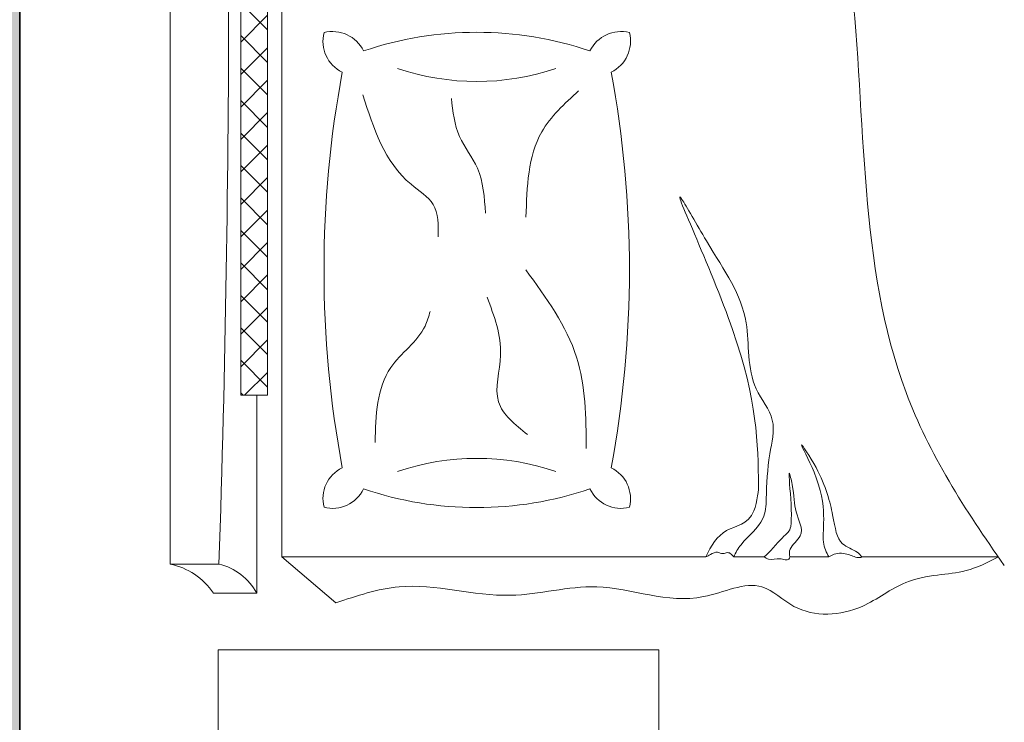
# Model space of a CAD drawing. Units: inches. Extents: x 2083 to 3317, y 1141 to 2115.
# Tile 95 of 256: x 2236 to 2290, y 1894 to 1932. Entities that reach past the tile are written whole.
import ezdxf

# ---------------------------------------------------------------- set-up
doc = ezdxf.new("R2010")
doc.units = ezdxf.units.IN
for name, color, linetype, lineweight in [('A-FURN', 8, 'Continuous', 18), ('A-WALL', 7, 'Continuous', 35), ('www.cadblocksfree.com', 7, 'Continuous', 9)]:
    doc.layers.add(name, color=color, linetype=linetype, lineweight=lineweight)
doc.layers.add('A-WALL-PATT', color=251, linetype='Continuous', lineweight=13, true_color=0x636466)

# ---------------------------------------------------------------- blocks, each defined once
blk = doc.blocks.new('bed')
at = {"layer": 'www.cadblocksfree.com', "ltscale": 0.2}
h = blk.add_hatch(dxfattribs=at)
h.set_pattern_fill('ANSI37,_O', color=256, scale=0.393701)
h.set_pattern_definition([(45, (2420.7222, -262.9689), (-0.8838835, 0.8838835), []), (135, (2420.7222, -262.9689), (-0.8838835, -0.8838835), [])])
h.paths.add_polyline_path([(3417.573, 1472.402), (3372.192, 1472.402), (3372.192, 1470.941), (3417.573, 1470.941)])
for p, q in [((3363.002, 1473.586), (3363.002, 1476.249)), ((3372.192, 1472.402), (3417.573, 1472.402)), ((3372.192, 1470.941), (3372.192, 1472.402)), ((3372.192, 1470.941), (3417.573, 1470.941)), ((3363.387, 1470.154), (3360.883, 1467.22))]:
    blk.add_line(p, q, dxfattribs=at)
for points in [[(3426.763, 1476.249), (3363.002, 1476.249)], [(3361.418, 1473.886), (3361.418, 1471.524), (3372.192, 1471.524)], [(3426.379, 1449.413), (3426.379, 1470.154), (3363.387, 1470.154), (3363.387, 1447.076)], [(3363.387, 1445.539), (3363.387, 1443.892)], [(3363.387, 1442.495), (3363.387, 1440.369)], [(3363.387, 1438.564), (3363.387, 1431.137)]]:
    blk.add_lwpolyline(points, dxfattribs=at)
for centre, radius, start, end in [((3359.334, 1476.997), 3.744, 303.8271, 348.4775), ((3359.844, 1474.373), 3.255, 298.9176, 345.9939), ((3394.883, 2431.358), 958.303, 268.093559, 271.906441), ((3367.903, 1467.396), 1.87, 165.5166, 244.2099), ((3366.56, 1466.054), 1.87, 25.7901, 104.4834), ((3379.014, 1409.187), 58.677, 79.42346, 100.57654), ((3391.467, 1466.054), 1.87, 75.5166, 154.2099), ((3390.125, 1467.396), 1.87, 295.7901, 14.4834), ((3385.289, 1459.547), 19.215, 161.2852, 198.7148), ((3372.739, 1459.547), 19.215, 341.2852, 18.7148), ((3355.416, 1459.547), 13.338, 341.1598, 18.8402), ((3402.612, 1459.547), 13.338, 161.1598, 198.8402), ((3367.903, 1451.698), 1.87, 115.7901, 194.4834), ((3390.125, 1451.698), 1.87, 345.5166, 64.2099), ((3366.56, 1453.041), 1.87, 255.5166, 334.2099), ((3379.014, 1509.907), 58.677, 259.42346, 280.57654), ((3391.467, 1453.041), 1.87, 205.7901, 284.4834)]:
    blk.add_arc(centre, radius, start, end, dxfattribs=at)
for points, knots in [([(3360.883, 1467.22), (3361.272, 1466.08), (3362.328, 1462.983), (3360.73, 1458.154), (3362.389, 1452.621), (3360.35, 1448.139), (3362.429, 1444.241), (3360.039, 1441.931), (3360.256, 1438.678), (3362.05, 1436.545), (3362.42, 1434.517), (3362.566, 1432.758), (3363.096, 1431.712), (3363.387, 1431.137)], [0, 0, 0, 0, 3.550403, 9.643115, 14.356056, 20.206026, 23.427697, 25.46537, 29.172767, 31.884544, 33.668442, 35.237641, 37.145618, 37.145618, 37.145618, 37.145618]), ([(3388.545, 1465.744), (3386.719, 1465.161), (3384.357, 1464.407), (3382.678, 1461.635), (3381.454, 1461.638), (3380.813, 1461.64)], [0, 0, 0, 0, 5.530688, 7.154877, 8.940839, 8.940839, 8.940839, 8.940839]), ([(3369.625, 1465.083), (3371.104, 1465.041), (3373.625, 1464.969), (3375.264, 1462.52), (3376.483, 1462.165), (3376.755, 1462.086)], [0, 0, 0, 0, 4.163459, 7.093919, 7.934624, 7.934624, 7.934624, 7.934624]), ([(3388.358, 1460.927), (3387.639, 1460.846), (3386.254, 1460.689), (3384.483, 1459.224), (3382.96, 1459.127), (3382.112, 1459.073)], [0, 0, 0, 0, 2.127543, 4.10272, 6.58647, 6.58647, 6.58647, 6.58647]), ([(3370.049, 1456.774), (3370.592, 1457.459), (3371.713, 1458.876), (3374.682, 1457.893), (3376.505, 1458.594), (3377.525, 1458.985)], [0, 0, 0, 0, 2.388143, 4.935423, 8.166198, 8.166198, 8.166198, 8.166198]), ([(3369.287, 1453.579), (3370.996, 1453.599), (3374.587, 1453.639), (3377.497, 1455.762), (3379.021, 1456.874)], [0, 0, 0, 0, 5.002087, 10.507046, 10.507046, 10.507046, 10.507046]), ([(3388.77, 1453.995), (3388.068, 1454.761), (3386.268, 1456.726), (3383.544, 1456.811), (3381.881, 1456.863)], [0, 0, 0, 0, 3.013696, 7.735839, 7.735839, 7.735839, 7.735839]), ([(3367.269, 1444.201), (3369.575, 1444.23), (3373.917, 1444.284), (3385.471, 1449.8), (3379.558, 1446.493), (3376.808, 1444.477), (3372.948, 1444.924), (3370.926, 1443.14), (3368.771, 1443.702), (3367.359, 1443.752), (3366.554, 1443.781)], [0, 0, 0, 0, 8.61026, 16.221274, 18.843057, 23.804898, 27.440828, 29.356102, 31.203478, 33.650687, 33.650687, 33.650687, 33.650687]), ([(3363.387, 1447.076), (3363.429, 1446.99), (3363.529, 1446.784), (3363.731, 1446.461), (3363.506, 1446.154), (3363.665, 1445.905), (3363.559, 1445.673), (3363.444, 1445.584), (3363.387, 1445.539)], [0, 0, 0, 0, 0.293454, 0.701471, 1.003873, 1.254893, 1.47342, 1.69185, 1.69185, 1.69185, 1.69185]), ([(3363.387, 1447.076), (3363.991, 1446.782), (3365.084, 1446.124), (3365.119, 1444.371), (3367.129, 1444.191), (3367.269, 1444.201)], [0.0122268, 0.0122268, 0.0122268, 0.0122268, 0.0594721, 0.1062177, 0.134458, 0.134458, 0.134458, 0.134458]), ([(3366.554, 1443.781), (3366.17, 1443.775), (3365.174, 1443.901), (3364.4, 1444.957), (3363.626, 1445.461), (3363.387, 1445.539)], [0.15648839, 0.15648839, 0.15648839, 0.15648839, 0.18439755, 0.23137648, 0.25059846, 0.25059846, 0.25059846, 0.25059846]), ([(3363.387, 1443.892), (3363.335, 1443.815), (3363.165, 1443.56), (3363.346, 1443.124), (3363.233, 1442.791), (3363.225, 1442.533), (3363.341, 1442.506), (3363.387, 1442.495)], [0, 0, 0, 0, 0.27176, 0.887321, 1.189132, 1.388142, 1.515331, 1.515331, 1.515331, 1.515331]), ([(3363.387, 1443.892), (3363.631, 1443.61), (3364.671, 1442.733), (3364.886, 1442.149), (3369.073, 1442.744), (3366.773, 1442.243), (3365.832, 1442.298), (3364.615, 1441.552), (3363.961, 1442.542), (3363.537, 1442.524), (3363.387, 1442.495)], [0.0595743, 0.0595743, 0.0595743, 0.0595743, 0.0807529, 0.1037415, 0.1697201, 0.1760361, 0.2071372, 0.2404744, 0.2623409, 0.2736605, 0.2736605, 0.2736605, 0.2736605]), ([(3362.928, 1430.813), (3365.944, 1432.958), (3375.455, 1438.993), (3392.12, 1438.03), (3404.249, 1440.73), (3408.408, 1442.961)], [0.102872, 0.102872, 0.102872, 0.102872, 0.37972, 0.957702, 1.313793, 1.313793, 1.313793, 1.313793]), ([(3363.387, 1440.369), (3363.634, 1440.51), (3364.527, 1440.899), (3366.485, 1440.246), (3370.203, 1442.295), (3367.731, 1440.636), (3365.42, 1440.07), (3364.035, 1439.913), (3363.795, 1438.935), (3363.482, 1438.64), (3363.387, 1438.564)], [0.013856, 0.013856, 0.013856, 0.013856, 0.0348738, 0.0888667, 0.1078792, 0.1267378, 0.158714, 0.1937575, 0.2174868, 0.2267221, 0.2267221, 0.2267221, 0.2267221]), ([(3363.387, 1440.369), (3363.445, 1440.274), (3363.571, 1440.065), (3363.607, 1439.678), (3363.531, 1439.31), (3363.405, 1439.003), (3363.329, 1438.751), (3363.372, 1438.611), (3363.387, 1438.564)], [0, 0, 0, 0, 0.329977, 0.725302, 1.129072, 1.442831, 1.734218, 1.878348, 1.878348, 1.878348, 1.878348])]:
    blk.add_open_spline(points, degree=3, knots=knots, dxfattribs=at)

msp = doc.modelspace()

# ---------------------------------------------------------------- hatches: boundary and pattern name
at = {"layer": 'A-WALL-PATT'}
h = msp.add_hatch(color=256, dxfattribs=at)
h.dxf.hatch_style = 1
h.paths.add_polyline_path([(3126.96, 2020.761), (2748.96, 2020.761), (2604.96, 2020.761), (2226.96, 2020.761), (2226.96, 1702.761), (2466.96, 1702.761), (2466.96, 1582.761), (2418.96, 1582.761), (2418.96, 1477.761), (2226.96, 1477.761), (2226.96, 1263.261), (2544.96, 1263.261), (2544.96, 1411.761), (2604.96, 1411.761), (2685.96, 1411.761), (2685.96, 1420.761), (2604.96, 1420.761), (2604.96, 1573.761), (2604.96, 1702.761), (2604.96, 2011.761), (2748.96, 2011.761), (2748.96, 1702.761), (2862.96, 1702.761), (2862.96, 1621.761), (2871.96, 1621.761), (2871.96, 1702.761), (2883.96, 1702.761), (2883.96, 1706.939, -0.026459), (2883.96, 1711.761), (2757.96, 1711.761), (2757.96, 1807.761), (2787.96, 1807.761), (2787.96, 1812.261), (2757.96, 1812.261), (2757.96, 2011.761), (2877.96, 2011.761), (2877.96, 1812.261), (2847.96, 1812.261), (2847.96, 1807.761), (2889.836, 1807.761), (2889.836, 1812.261), (2882.46, 1812.261), (2882.46, 2011.761), (3117.96, 2011.761), (3117.96, 1812.261), (2937.836, 1812.261), (2937.836, 1807.761), (2995.71, 1807.761), (2995.71, 1796.118), (3000.21, 1796.118), (3000.21, 1807.761), (3117.96, 1807.761), (3117.96, 1711.761), (3000.21, 1711.761), (3000.21, 1760.118), (2998.573, 1760.118, -0.020711), (2995.71, 1760.118), (2995.71, 1711.761), (2931.96, 1711.761), (2931.96, 1702.761), (3126.96, 1702.761)])
h.paths.add_polyline_path([(2471.46, 2011.761), (2471.46, 1810.011), (2462.717, 1810.011), (2462.717, 1805.511), (2505.96, 1805.511), (2505.96, 1810.011), (2475.96, 1810.011), (2475.96, 2011.761), (2595.96, 2011.761), (2595.96, 1810.011), (2565.96, 1810.011), (2565.96, 1805.511), (2595.96, 1805.511), (2595.96, 1711.761), (2235.96, 1711.761), (2235.96, 1805.511), (2353.71, 1805.511), (2353.71, 1796.054), (2358.21, 1796.054), (2358.21, 1805.511), (2414.717, 1805.511), (2414.717, 1810.011), (2235.96, 1810.011), (2235.96, 2011.761)], flags=16)
h.paths.add_polyline_path([(2270.205, 1994.61), (2270.205, 1970.61), (2246.205, 1970.61), (2246.205, 1994.61)], flags=0)
edge = h.paths.add_edge_path(flags=0)
edge.add_ellipse((2332.027, 1899.798), major_axis=(-3.043, 3.043), ratio=0.168252, start_angle=-161.3322, end_angle=-156.3071, ccw=False)
edge.add_ellipse((2333.082, 1898.744), major_axis=(-1.055, 1.055), ratio=0.453532, start_angle=-123.371, end_angle=-94.1591)
edge = h.paths.add_edge_path(flags=0)
edge.add_ellipse((2332.027, 1968.876), major_axis=(3.043, 3.043), ratio=0.168252, start_angle=18.6678, end_angle=23.6929)
edge.add_spline(control_points=[(2332.926, 1970.691), (2332.227, 1970.336), (2330.894, 1969.659), (2328.413, 1970.932), (2327.204, 1967.749), (2324.71, 1969.956), (2322.533, 1967.012), (2320.013, 1971.296), (2317.68, 1968.158), (2316.041, 1967.102), (2315.427, 1966.81)], knot_values=[0, 0, 0, 0, 2.267059, 4.324559, 6.685584, 8.878641, 11.121502, 14.300359, 17.755284, 19.732645, 19.732645, 19.732645, 19.732645], degree=3, periodic=0)
edge.add_ellipse((2332.027, 1968.876), major_axis=(3.043, 3.043), ratio=0.168252, start_angle=18.6678, end_angle=23.6929, ccw=False)
edge.add_ellipse((2333.082, 1969.931), major_axis=(1.055, 1.055), ratio=0.453532, start_angle=56.629, end_angle=85.8409, ccw=False)
edge = h.paths.add_edge_path(flags=0)
edge.add_spline(control_points=[(2296.428, 1967.988), (2293.628, 1965.336), (2287.704, 1959.727), (2299.744, 1949.996), (2294.533, 1935.669), (2290.573, 1920.604), (2293.394, 1909.974), (2296.185, 1904.967)], knot_values=[0.099185, 0.099185, 0.099185, 0.099185, 0.345301, 0.619822, 0.982653, 1.386093, 1.810555, 1.810555, 1.810555, 1.810555], degree=3, periodic=0)
edge.add_spline(control_points=[(2296.185, 1904.967), (2297.384, 1902.619), (2298.001, 1901.949), (2298.553, 1901.468)], knot_values=[0.006246, 0.006246, 0.006246, 0.006246, 0.055476, 0.055476, 0.055476, 0.055476], degree=3, periodic=0)
edge.add_spline(control_points=[(2298.553, 1901.468), (2297.259, 1900.923), (2295.225, 1900.232), (2293.06, 1900.614), (2292.101, 1900.788), (2292.09, 1900.791)], knot_values=[0.312835, 0.312835, 0.312835, 0.312835, 0.40178, 0.474987, 0.475903, 0.475903, 0.475903, 0.475903], degree=3, periodic=0)
edge.add_arc((2292.794, 1904.664), 3.937, 215.4209, 259.6982, ccw=False)
edge.add_spline(control_points=[(2289.585, 1902.382), (2289.477, 1902.535), (2289.368, 1902.688), (2289.261, 1902.841)], knot_values=[0.102872, 0.102872, 0.102872, 0.102872, 0.116896, 0.116896, 0.116896, 0.116896], degree=3, periodic=0)
edge.add_spline(control_points=[(2289.261, 1902.841), (2288.687, 1902.55), (2287.64, 1902.02), (2285.881, 1901.874), (2283.853, 1901.504), (2281.72, 1899.711), (2278.467, 1899.493), (2276.157, 1901.883), (2272.259, 1899.804), (2267.778, 1901.843), (2262.244, 1900.184), (2257.415, 1901.782), (2254.318, 1900.726), (2253.178, 1900.337)], knot_values=[0, 0, 0, 0, 1.907977, 3.477176, 5.261074, 7.972851, 11.680248, 13.717921, 16.939592, 22.789562, 27.502503, 33.595215, 37.145618, 37.145618, 37.145618, 37.145618], degree=3, periodic=0)
edge.add_line((2253.178, 1900.337), (2250.244, 1902.841))
edge.add_line((2250.244, 1902.841), (2250.244, 1965.833))
edge.add_line((2250.244, 1965.833), (2253.178, 1968.337))
edge.add_spline(control_points=[(2253.178, 1968.337), (2254.318, 1967.948), (2257.415, 1966.892), (2262.244, 1968.49), (2267.778, 1966.831), (2271.527, 1968.537), (2273.876, 1967.828), (2274.207, 1967.728)], knot_values=[0, 0, 0, 0, 0.09018, 0.244935, 0.364644, 0.513233, 0.537855, 0.537855, 0.537855, 0.537855], degree=3, periodic=0)
edge.add_arc((2274.353, 1963.793), 3.937, 72.0511, 92.1279, ccw=False)
edge.add_arc((2281.297, 1985.23), 18.596, 252.0511, 288.5657)
edge.add_arc((2292.317, 1956.029), 12.646, 71.0268, 113.7782, ccw=False)
edge = h.paths.add_edge_path(flags=0)
edge.add_spline(control_points=[(2274.899, 1951.856), (2275.066, 1951.617), (2275.233, 1951.377), (2275.398, 1951.136)], knot_values=[1.409916, 1.409916, 1.409916, 1.409916, 1.43159, 1.43159, 1.43159, 1.43159], degree=3, periodic=0)
edge.add_spline(control_points=[(2275.398, 1951.136), (2275.792, 1950.562), (2276.179, 1949.984), (2276.546, 1949.397)], knot_values=[1.358238, 1.358238, 1.358238, 1.358238, 1.409916, 1.409916, 1.409916, 1.409916], degree=3, periodic=0)
edge.add_line((2276.546, 1949.397), (2277.437, 1947.862))
edge.add_spline(control_points=[(2277.437, 1947.862), (2276.304, 1945.673), (2274.64, 1942.427), (2274.632, 1938.094), (2272.799, 1930.852), (2274.356, 1943.897), (2275.948, 1947.923), (2276.546, 1949.397)], knot_values=[0.005632, 0.005632, 0.005632, 0.005632, 0.186014, 0.266002, 0.357087, 0.59639, 0.739732, 0.739732, 0.739732, 0.739732], degree=3, periodic=0)
edge.add_spline(control_points=[(2276.546, 1949.397), (2276.179, 1949.984), (2275.792, 1950.562), (2275.398, 1951.136)], knot_values=[1.358238, 1.358238, 1.358238, 1.358238, 1.409916, 1.409916, 1.409916, 1.409916], degree=3, periodic=0)
edge.add_spline(control_points=[(2275.398, 1951.136), (2274.943, 1950.08), (2274.208, 1948.025), (2273.935, 1944.851), (2272.469, 1937.627), (2273.466, 1945.696), (2274.701, 1951.059), (2274.899, 1951.856)], knot_values=[0.104364, 0.104364, 0.104364, 0.104364, 0.189636, 0.269624, 0.36071, 0.600013, 0.644622, 0.644622, 0.644622, 0.644622], degree=3, periodic=0)
h.paths.add_polyline_path([(2269.168, 1963.128, -0.357527), (2268.171, 1960.976, -0.092561), (2268.171, 1939.436, -0.357527), (2269.168, 1937.285, -0.357527), (2267.016, 1938.282, -0.164785), (2254.686, 1938.282, -0.357527), (2252.534, 1937.285, -0.357527), (2253.531, 1939.436, -0.092561), (2253.531, 1960.976, -0.357527), (2252.534, 1963.128, -0.357527), (2254.686, 1962.131, -0.164785), (2267.016, 1962.131, -0.357527)], flags=0)
h.paths.add_polyline_path([(2248.874, 1967.802), (2248.874, 1957.028), (2249.458, 1957.028), (2249.458, 1911.647), (2248.874, 1911.647), (2248.874, 1900.873), (2246.512, 1900.873, 0.197327), (2244.15, 1902.457), (2244.15, 1966.218, 0.197327), (2246.512, 1967.802)], flags=0)
h.paths.add_polyline_path([(2269.168, 1931.389, -0.357527), (2268.171, 1929.238, -0.092561), (2268.171, 1907.698, -0.357527), (2269.168, 1905.547, -0.357527), (2267.016, 1906.544, -0.164785), (2254.686, 1906.544, -0.357527), (2252.534, 1905.547, -0.357527), (2253.531, 1907.698, -0.092561), (2253.531, 1929.238, -0.357527), (2252.534, 1931.389, -0.357527), (2254.686, 1930.392, -0.164785), (2267.016, 1930.392, -0.357527)], flags=0)
edge = h.paths.add_edge_path(flags=0)
edge.add_spline(control_points=[(2276.197, 1906.724), (2276.168, 1909.029), (2276.114, 1913.372), (2270.598, 1924.925), (2273.905, 1919.013), (2275.922, 1916.262), (2275.475, 1912.402), (2277.258, 1910.381), (2276.696, 1908.225), (2276.646, 1906.813), (2276.618, 1906.008)], knot_values=[0, 0, 0, 0, 8.61026, 16.221274, 18.843057, 23.804898, 27.440828, 29.356102, 31.203478, 33.650687, 33.650687, 33.650687, 33.650687], degree=3, periodic=0)
edge.add_spline(control_points=[(2276.618, 1906.008), (2276.623, 1905.624), (2276.498, 1904.629), (2275.442, 1903.855), (2274.937, 1903.08), (2274.859, 1902.841)], knot_values=[0.156488, 0.156488, 0.156488, 0.156488, 0.184398, 0.231376, 0.250598, 0.250598, 0.250598, 0.250598], degree=3, periodic=0)
edge.add_line((2274.859, 1902.841), (2276.506, 1902.841))
edge.add_spline(control_points=[(2276.506, 1902.841), (2276.788, 1903.085), (2277.665, 1904.125), (2278.25, 1904.341), (2277.654, 1908.527), (2278.156, 1906.228), (2278.1, 1905.286), (2278.847, 1904.069), (2277.857, 1903.415), (2277.874, 1902.991), (2277.904, 1902.841)], knot_values=[0.059574, 0.059574, 0.059574, 0.059574, 0.080753, 0.103741, 0.16972, 0.176036, 0.207137, 0.240474, 0.262341, 0.27366, 0.27366, 0.27366, 0.27366], degree=3, periodic=0)
edge.add_line((2277.904, 1902.841), (2280.03, 1902.841))
edge.add_spline(control_points=[(2280.03, 1902.841), (2279.888, 1903.088), (2279.499, 1903.982), (2280.152, 1905.939), (2278.104, 1909.658), (2279.762, 1907.185), (2280.328, 1904.875), (2280.485, 1903.49), (2281.463, 1903.249), (2281.758, 1902.936), (2281.834, 1902.841)], knot_values=[0.013856, 0.013856, 0.013856, 0.013856, 0.034874, 0.088867, 0.107879, 0.126738, 0.158714, 0.193757, 0.217487, 0.226722, 0.226722, 0.226722, 0.226722], degree=3, periodic=0)
edge.add_spline(control_points=[(2281.834, 1902.841), (2281.788, 1902.827), (2281.647, 1902.783), (2281.396, 1902.859), (2281.088, 1902.985), (2280.721, 1903.061), (2280.333, 1903.026), (2280.125, 1902.899), (2280.03, 1902.841)], knot_values=[0, 0, 0, 0, 0.14413, 0.435517, 0.749276, 1.153046, 1.548371, 1.878348, 1.878348, 1.878348, 1.878348], degree=3, periodic=0)
edge.add_line((2280.03, 1902.841), (2277.904, 1902.841))
edge.add_spline(control_points=[(2277.904, 1902.841), (2277.893, 1902.796), (2277.865, 1902.68), (2277.607, 1902.687), (2277.274, 1902.801), (2276.838, 1902.62), (2276.584, 1902.789), (2276.506, 1902.841)], knot_values=[0, 0, 0, 0, 0.127189, 0.326199, 0.628009, 1.24357, 1.515331, 1.515331, 1.515331, 1.515331], degree=3, periodic=0)
edge.add_line((2276.506, 1902.841), (2274.859, 1902.841))
edge.add_spline(control_points=[(2274.859, 1902.841), (2274.814, 1902.899), (2274.725, 1903.013), (2274.493, 1903.119), (2274.244, 1902.961), (2273.937, 1903.185), (2273.614, 1902.983), (2273.408, 1902.883), (2273.322, 1902.841)], knot_values=[0, 0, 0, 0, 0.21843, 0.436957, 0.687977, 0.990379, 1.398396, 1.69185, 1.69185, 1.69185, 1.69185], degree=3, periodic=0)
edge.add_spline(control_points=[(2273.322, 1902.841), (2273.617, 1903.446), (2274.274, 1904.538), (2276.027, 1904.574), (2276.207, 1906.584), (2276.197, 1906.724)], knot_values=[0.012227, 0.012227, 0.012227, 0.012227, 0.059472, 0.106218, 0.134458, 0.134458, 0.134458, 0.134458], degree=3, periodic=0)
h.paths.add_polyline_path([(2270.776, 1897.79), (2270.776, 1873.79), (2246.776, 1873.79), (2246.776, 1897.79)], flags=0)
h.paths.add_polyline_path([(2353.71, 1760.005), (2353.71, 1760.054), (2358.21, 1760.054, -0.033729)], flags=0)
h.paths.add_polyline_path([(2321.819, 1737.529), (2341.995, 1737.529, -0.414214), (2343.203, 1736.321), (2343.203, 1721.021, -0.414214), (2341.995, 1719.813), (2321.819, 1719.813, -0.414214), (2320.611, 1721.021), (2320.611, 1736.321, -0.414214)], flags=0)
h.paths.add_polyline_path([(2324.235, 1736.321), (2339.579, 1736.321, -0.414214), (2341.995, 1733.905), (2341.995, 1725.45, -0.414214), (2339.579, 1723.034), (2333.681, 1723.034), (2333.845, 1722.045, -0.870646), (2335.425, 1721.826, -0.767327), (2333.923, 1721.423), (2331.291, 1721.423, -0.767327), (2329.788, 1721.826, -0.870646), (2331.368, 1722.045), (2331.533, 1723.034), (2324.235, 1723.034, -0.414214), (2321.819, 1725.45), (2321.819, 1733.905, -0.414214)], flags=0)
h.paths.add_polyline_path([(2570.484, 1928.615), (2589.684, 1928.615), (2590.169, 1928.615), (2590.169, 1904.993), (2570.484, 1904.993)], flags=0)
h.paths.add_polyline_path([(2574.447, 1927.264, -1), (2572.829, 1927.264, -1)], flags=0)
h.paths.add_polyline_path([(2573.09, 1926.941), (2573.925, 1927.776), (2574.148, 1927.553), (2573.313, 1926.718)], flags=0)
h.paths.add_polyline_path([(2578.779, 1919.73, -1), (2571.592, 1919.73, -1)], flags=0)
h.paths.add_polyline_path([(2578.385, 1919.73, -1), (2571.985, 1919.73, -1)], flags=0)
h.paths.add_polyline_path([(2331.596, 1729.476, -1), (2333.618, 1729.476, -1)], flags=0)
h.paths.add_polyline_path([(2578.034, 1927.264, -1), (2576.416, 1927.264, -1)], flags=0)
h.paths.add_polyline_path([(2576.689, 1927.531), (2576.912, 1927.754), (2577.747, 1926.919), (2577.524, 1926.696)], flags=0)
h.paths.add_polyline_path([(2578.139, 1909.86, -1), (2572.232, 1909.86, -1)], flags=0)
h.paths.add_polyline_path([(2577.745, 1909.86, -1), (2572.625, 1909.86, -1)], flags=0)
h.paths.add_polyline_path([(2583.798, 1927.264, -1), (2582.179, 1927.264, -1)], flags=0)
h.paths.add_polyline_path([(2582.719, 1927.754), (2583.554, 1926.919), (2583.331, 1926.696), (2582.496, 1927.531)], flags=0)
h.paths.add_polyline_path([(2582.496, 1927.531), (2582.719, 1927.754), (2583.554, 1926.919), (2583.331, 1926.696)], flags=0)
h.paths.add_polyline_path([(2587.739, 1920.53, -1), (2581.832, 1920.53, -1)], flags=0)
h.paths.add_polyline_path([(2587.345, 1920.53, -1), (2582.225, 1920.53, -1)], flags=0)
h.paths.add_polyline_path([(2587.385, 1927.264, -1), (2585.766, 1927.264, -1)], flags=0)
h.paths.add_polyline_path([(2586.082, 1926.98), (2586.917, 1927.815), (2587.14, 1927.593), (2586.305, 1926.758)], flags=0)
h.paths.add_polyline_path([(2588.379, 1910.66, -1), (2581.192, 1910.66, -1)], flags=0)
h.paths.add_polyline_path([(2587.985, 1910.66, -1), (2581.585, 1910.66, -1)], flags=0)
h.paths.add_polyline_path([(2417.168, 1729.478), (2437.344, 1729.478, -0.414214), (2438.552, 1728.27), (2438.552, 1712.969, -0.414214), (2437.344, 1711.761), (2417.168, 1711.761, -0.414214), (2415.96, 1712.969), (2415.96, 1728.27, -0.414214)], flags=0)
h.paths.add_polyline_path([(2419.584, 1728.27), (2434.928, 1728.27, -0.414214), (2437.344, 1725.854), (2437.344, 1717.398, -0.414214), (2434.928, 1714.983), (2429.029, 1714.983), (2429.194, 1713.994, -0.870646), (2430.774, 1713.775, -0.767327), (2429.271, 1713.372), (2426.64, 1713.372, -0.767327), (2425.137, 1713.775, -0.870646), (2426.717, 1713.994), (2426.882, 1714.983), (2419.584, 1714.983, -0.414214), (2417.168, 1717.398), (2417.168, 1725.854, -0.414214)], flags=0)
h.paths.add_polyline_path([(2419.584, 1728.27), (2434.928, 1728.27, -0.414214), (2437.344, 1725.854), (2437.344, 1717.398, -0.414214), (2434.928, 1714.983), (2429.029, 1714.983), (2428.358, 1719.009), (2427.553, 1719.009), (2426.882, 1714.983), (2419.584, 1714.983, -0.414214), (2417.168, 1717.398), (2417.168, 1725.854, -0.414214)], flags=0)
h.paths.add_polyline_path([(2426.944, 1721.425, -1), (2428.967, 1721.425, -1)], flags=0)
h.paths.add_polyline_path([(2475.96, 1702.761), (2595.96, 1702.761), (2595.96, 1582.761), (2475.96, 1582.761)], flags=16)
h.paths.add_polyline_path([(2427.96, 1573.761), (2595.96, 1573.761), (2595.96, 1468.761), (2595.96, 1420.761), (2384.46, 1420.761), (2384.46, 1468.761), (2427.96, 1468.761)], flags=16)
h.paths.add_polyline_path([(2379.96, 1468.761), (2379.96, 1420.761), (2235.96, 1420.761), (2235.96, 1468.761)], flags=16)
h.paths.add_polyline_path([(2317.816, 1466.696), (2337.992, 1466.696, -0.414214), (2339.2, 1465.488), (2339.2, 1450.187, -0.414214), (2337.992, 1448.979), (2317.816, 1448.979, -0.414214), (2316.608, 1450.187), (2316.608, 1465.488, -0.414214)], flags=0)
h.paths.add_polyline_path([(2320.232, 1465.488), (2335.576, 1465.488, -0.414214), (2337.992, 1463.072), (2337.992, 1454.616, -0.414214), (2335.576, 1452.2), (2329.677, 1452.2), (2329.842, 1451.212, -0.870646), (2331.422, 1450.992, -0.767327), (2329.92, 1450.59), (2327.288, 1450.59, -0.767327), (2325.785, 1450.992, -0.870646), (2327.365, 1451.212), (2327.53, 1452.2), (2320.232, 1452.2, -0.414214), (2317.816, 1454.616), (2317.816, 1463.072, -0.414214)], flags=0)
h.paths.add_polyline_path([(2320.232, 1465.488), (2335.576, 1465.488, -0.414214), (2337.992, 1463.072), (2337.992, 1454.616, -0.414214), (2335.576, 1452.2), (2329.677, 1452.2), (2329.006, 1456.227), (2328.201, 1456.227), (2327.53, 1452.2), (2320.232, 1452.2, -0.414214), (2317.816, 1454.616), (2317.816, 1463.072, -0.414214)], flags=0)
h.paths.add_polyline_path([(2327.593, 1458.643, -1), (2329.615, 1458.643, -1)], flags=0)
h.paths.add_polyline_path([(2244.412, 1433.34), (2241.921, 1433.34, -0.414214), (2240.018, 1435.244), (2240.018, 1440.953, -0.414211), (2241.921, 1442.856), (2244.412, 1442.856, -1.976472)], flags=0)
h.paths.add_polyline_path([(2245.357, 1434.398, -0.414214), (2245.357, 1441.799, -2.144098)], flags=0)
h.paths.add_polyline_path([(2535.96, 1416.261), (2535.96, 1272.261), (2235.96, 1272.261), (2235.96, 1416.261)], flags=16)
h.paths.add_polyline_path([(2260.12, 1384.293), (2260.12, 1362.039), (2237.865, 1362.039), (2237.865, 1384.293)], flags=0)
edge = h.paths.add_edge_path(flags=0)
edge.add_line((2318.252, 1362.093), (2318.146, 1362.001))
edge.add_ellipse((2317.445, 1360.431), major_axis=(2.822, 2.822), ratio=0.168252, start_angle=18.6678, end_angle=20.9481, ccw=False)
edge.add_ellipse((2318.423, 1361.409), major_axis=(0.978, 0.978), ratio=0.453532, start_angle=56.629, end_angle=70.2262, ccw=False)
edge = h.paths.add_edge_path(flags=0)
edge.add_line((2319.107, 1295.571), (2319.015, 1295.677))
edge.add_ellipse((2317.445, 1296.378), major_axis=(-2.822, 2.822), ratio=0.168252, start_angle=-161.3322, end_angle=-159.0519, ccw=False)
edge.add_ellipse((2318.423, 1295.4), major_axis=(-0.978, 0.978), ratio=0.453532, start_angle=-123.371, end_angle=-109.7738)
edge = h.paths.add_edge_path(flags=0)
edge.add_spline(control_points=[(2284.21, 1301.17), (2284.581, 1300.445), (2284.891, 1299.892), (2285.16, 1299.461)], knot_values=[0.039066, 0.039066, 0.039066, 0.039066, 0.055476, 0.055476, 0.055476, 0.055476], degree=3, periodic=0)
edge.add_line((2285.16, 1299.461), (2284.21, 1301.17))
edge = h.paths.add_edge_path(flags=0)
edge.add_line((2280.412, 1297.298), (2283.37, 1297.036))
edge.add_line((2283.37, 1297.036), (2286.406, 1297.926))
edge.add_spline(control_points=[(2286.406, 1297.926), (2285.305, 1297.463), (2284.345, 1297.129), (2283.37, 1297.036)], knot_values=[0.394369, 0.394369, 0.394369, 0.394369, 0.475903, 0.475903, 0.475903, 0.475903], degree=3, periodic=0)
edge.add_spline(control_points=[(2283.37, 1297.036), (2283.281, 1297.028), (2282.316, 1296.957), (2281.313, 1297.134), (2280.423, 1297.296), (2280.412, 1297.298)], knot_values=[0.312835, 0.312835, 0.312835, 0.312835, 0.320246, 0.393453, 0.394369, 0.394369, 0.394369, 0.394369], degree=3, periodic=0)
edge = h.paths.add_edge_path(flags=0)
edge.add_line((2284.436, 1359.607), (2280.446, 1355.328))
edge.add_line((2280.446, 1355.328), (2279.58, 1351.018))
edge.add_line((2279.58, 1351.018), (2282.413, 1346.58))
edge.add_spline(control_points=[(2282.413, 1346.58), (2283.153, 1345.589), (2284.253, 1344.029), (2284.801, 1342.387), (2284.935, 1341.806)], knot_values=[1.240098, 1.240098, 1.240098, 1.240098, 1.332892, 1.382712, 1.382712, 1.382712, 1.382712], degree=3, periodic=0)
edge.add_spline(control_points=[(2284.935, 1341.806), (2285.319, 1340.141), (2285.233, 1338.409), (2284.91, 1336.654)], knot_values=[1.097484, 1.097484, 1.097484, 1.097484, 1.240098, 1.240098, 1.240098, 1.240098], degree=3, periodic=0)
edge.add_spline(control_points=[(2284.91, 1336.654), (2284.587, 1334.899), (2284.027, 1333.12), (2283.463, 1331.361)], knot_values=[0.95487, 0.95487, 0.95487, 0.95487, 1.097484, 1.097484, 1.097484, 1.097484], degree=3, periodic=0)
edge.add_line((2283.463, 1331.361), (2281.89, 1326.153))
edge.add_line((2281.89, 1326.153), (2280.756, 1321.056))
edge.add_line((2280.756, 1321.056), (2280.299, 1316.002))
edge.add_line((2280.299, 1316.002), (2280.716, 1310.95))
edge.add_line((2280.716, 1310.95), (2282.028, 1305.972))
edge.add_line((2282.028, 1305.972), (2284.21, 1301.17))
edge.add_spline(control_points=[(2284.21, 1301.17), (2283.341, 1302.73), (2282.612, 1304.336), (2282.028, 1305.972)], knot_values=[0.099185, 0.099185, 0.099185, 0.099185, 0.241799, 0.241799, 0.241799, 0.241799], degree=3, periodic=0)
edge.add_spline(control_points=[(2282.028, 1305.972), (2281.444, 1307.608), (2281.005, 1309.273), (2280.716, 1310.95)], knot_values=[0.241799, 0.241799, 0.241799, 0.241799, 0.384413, 0.384413, 0.384413, 0.384413], degree=3, periodic=0)
edge.add_spline(control_points=[(2280.716, 1310.95), (2280.433, 1312.588), (2280.289, 1314.277), (2280.299, 1315.962), (2280.299, 1316.002)], knot_values=[0.384413, 0.384413, 0.384413, 0.384413, 0.523647, 0.527028, 0.527028, 0.527028, 0.527028], degree=3, periodic=0)
edge.add_spline(control_points=[(2280.299, 1316.002), (2280.312, 1317.687), (2280.478, 1319.368), (2280.756, 1321.056)], knot_values=[0.527028, 0.527028, 0.527028, 0.527028, 0.669642, 0.669642, 0.669642, 0.669642], degree=3, periodic=0)
edge.add_spline(control_points=[(2280.756, 1321.056), (2281.035, 1322.744), (2281.426, 1324.44), (2281.89, 1326.153)], knot_values=[0.669642, 0.669642, 0.669642, 0.669642, 0.812256, 0.812256, 0.812256, 0.812256], degree=3, periodic=0)
edge.add_spline(control_points=[(2281.89, 1326.153), (2282.264, 1327.533), (2282.788, 1329.262), (2283.353, 1331.018), (2283.463, 1331.361)], knot_values=[0.812256, 0.812256, 0.812256, 0.812256, 0.927087, 0.95487, 0.95487, 0.95487, 0.95487], degree=3, periodic=0)
edge.add_line((2283.463, 1331.361), (2284.91, 1336.654))
edge.add_line((2284.91, 1336.654), (2284.935, 1341.806))
edge.add_line((2284.935, 1341.806), (2282.413, 1346.58))
edge.add_spline(control_points=[(2282.413, 1346.58), (2281.275, 1348.104), (2280.078, 1349.57), (2279.58, 1351.018)], knot_values=[1.382712, 1.382712, 1.382712, 1.382712, 1.525326, 1.525326, 1.525326, 1.525326], degree=3, periodic=0)
edge.add_spline(control_points=[(2279.58, 1351.018), (2279.443, 1351.415), (2279.136, 1352.857), (2279.735, 1354.29), (2280.446, 1355.328)], knot_values=[1.525326, 1.525326, 1.525326, 1.525326, 1.564439, 1.667941, 1.667941, 1.667941, 1.667941], degree=3, periodic=0)
edge.add_spline(control_points=[(2280.446, 1355.328), (2281.426, 1356.758), (2282.931, 1358.183), (2284.436, 1359.607)], knot_values=[1.667941, 1.667941, 1.667941, 1.667941, 1.810555, 1.810555, 1.810555, 1.810555], degree=3, periodic=0)
edge.add_arc((2280.623, 1348.518), 11.726, 71.0268, 113.7782)
edge.add_arc((2270.405, 1375.595), 17.244, 252.0511, 288.5657, ccw=False)
edge.add_arc((2263.966, 1355.718), 3.651, 72.0511, 92.1279)
edge.add_arc((2263.966, 1355.718), 3.651, 92.1279, 177.9851)
edge.add_spline(control_points=[(2260.318, 1355.846), (2260.26, 1354.221), (2260.551, 1350.187), (2262.999, 1346.766), (2264.473, 1344.649)], knot_values=[1.43159, 1.43159, 1.43159, 1.43159, 1.564144, 1.770695, 1.770695, 1.770695, 1.770695], degree=3, periodic=0)
edge.add_line((2264.473, 1344.649), (2264.936, 1343.983))
edge.add_spline(control_points=[(2263.801, 1340.248), (2263.843, 1340.514), (2264.067, 1341.756), (2264.513, 1343.002), (2264.935, 1343.981)], knot_values=[0.53657, 0.53657, 0.53657, 0.53657, 0.559349, 0.644622, 0.644622, 0.644622, 0.644622], degree=3, periodic=0)
edge.add_spline(control_points=[(2264.935, 1343.981), (2265.118, 1343.715), (2265.299, 1343.448), (2265.477, 1343.179)], knot_values=[1.384077, 1.384077, 1.384077, 1.384077, 1.409916, 1.409916, 1.409916, 1.409916], degree=3, periodic=0)
edge.add_spline(control_points=[(2265.477, 1343.179), (2265.655, 1342.911), (2265.829, 1342.641), (2265.999, 1342.369)], knot_values=[1.358238, 1.358238, 1.358238, 1.358238, 1.384077, 1.384077, 1.384077, 1.384077], degree=3, periodic=0)
edge.add_line((2265.999, 1342.369), (2266.826, 1340.946))
edge.add_spline(control_points=[(2266.826, 1340.946), (2268.894, 1337.09), (2271.398, 1325.843), (2270.516, 1310.569), (2275.919, 1301.861), (2277.79, 1299.199)], knot_values=[0.116896, 0.116896, 0.116896, 0.116896, 0.472987, 1.050969, 1.313793, 1.313793, 1.313793, 1.313793], degree=3, periodic=0)
edge.add_spline(control_points=[(2277.79, 1299.199), (2277.839, 1299.128), (2277.889, 1299.057), (2277.94, 1298.987)], knot_values=[0.109884, 0.109884, 0.109884, 0.109884, 0.116896, 0.116896, 0.116896, 0.116896], degree=3, periodic=0)
edge.add_line((2277.94, 1298.987), (2277.789, 1299.199))
edge.add_spline(control_points=[(2277.789, 1299.199), (2277.257, 1298.929), (2276.286, 1298.438), (2275.039, 1298.334), (2274.383, 1298.239), (2274.215, 1298.209)], knot_values=[33.12187, 33.12187, 33.12187, 33.12187, 35.029056, 36.598255, 37.144827, 37.144827, 37.144827, 37.144827], degree=3, periodic=0)
edge.add_line((2274.215, 1298.209), (2273.073, 1297.893))
edge.add_spline(control_points=[(2273.073, 1297.893), (2272.323, 1297.58), (2271.039, 1296.511), (2269.248, 1296.226), (2268.423, 1296.375)], knot_values=[26.532584, 26.532584, 26.532584, 26.532584, 29.198919, 31.839101, 31.839101, 31.839101, 31.839101], degree=3, periodic=0)
edge.add_line((2268.423, 1296.375), (2263.879, 1297.458))
edge.add_spline(control_points=[(2263.879, 1297.458), (2263.556, 1297.359), (2261.86, 1296.839), (2260.239, 1297.282), (2258.933, 1297.516)], knot_values=[15.919551, 15.919551, 15.919551, 15.919551, 16.939592, 21.226067, 21.226067, 21.226067, 21.226067], degree=3, periodic=0)
edge.add_line((2258.933, 1297.516), (2254.055, 1297.329))
edge.add_spline(control_points=[(2254.055, 1297.329), (2253.756, 1297.296), (2252.114, 1297.165), (2250.462, 1297.544), (2249.13, 1297.668)], knot_values=[5.306517, 5.306517, 5.306517, 5.306517, 6.276435, 10.613034, 10.613034, 10.613034, 10.613034], degree=3, periodic=0)
edge.add_line((2249.13, 1297.668), (2244.332, 1296.878))
edge.add_line((2244.332, 1296.878), (2241.611, 1299.199))
edge.add_line((2241.611, 1299.199), (2241.611, 1357.609))
edge.add_line((2241.611, 1357.609), (2244.332, 1359.931))
edge.add_line((2244.332, 1359.931), (2252.729, 1359.543))
edge.add_spline(control_points=[(2252.729, 1359.543), (2252.871, 1359.546), (2253.306, 1359.548), (2253.74, 1359.514), (2254.032, 1359.482)], knot_values=[0.233291, 0.233291, 0.233291, 0.233291, 0.244935, 0.268927, 0.268927, 0.268927, 0.268927], degree=3, periodic=0)
edge.add_line((2254.032, 1359.482), (2259.587, 1359.416))
edge.add_spline(control_points=[(2259.587, 1359.416), (2260.677, 1359.629), (2262.073, 1359.897), (2263.524, 1359.459), (2263.83, 1359.366)], knot_values=[0.422516, 0.422516, 0.422516, 0.422516, 0.513233, 0.537855, 0.537855, 0.537855, 0.537855], degree=3, periodic=0)
edge.add_arc((2263.966, 1355.718), 3.651, 72.0511, 92.1279, ccw=False)
edge.add_arc((2270.405, 1375.595), 17.244, 252.0511, 288.5657)
edge.add_arc((2280.623, 1348.518), 11.726, 71.0268, 113.7782, ccw=False)
h.paths.add_polyline_path([(2240.341, 1359.435), (2240.341, 1349.444), (2240.882, 1349.444), (2240.882, 1307.365), (2240.341, 1307.365), (2240.341, 1297.374), (2238.15, 1297.374, 0.197327), (2235.96, 1298.843), (2235.96, 1357.966, 0.197327), (2238.15, 1359.435)], flags=0)
h.paths.add_polyline_path([(2259.158, 1355.101, -0.357527), (2258.233, 1353.106, -0.092561), (2258.233, 1333.133, -0.357527), (2259.158, 1331.138, -0.357527), (2257.163, 1332.062, -0.164785), (2245.729, 1332.062, -0.357527), (2243.735, 1331.138, -0.357527), (2244.659, 1333.133, -0.092561), (2244.659, 1353.106, -0.357527), (2243.735, 1355.101, -0.357527), (2245.729, 1354.176, -0.164785), (2257.163, 1354.176, -0.357527)], flags=0)
edge = h.paths.add_edge_path(flags=0)
edge.add_line((2265.999, 1342.369), (2266.826, 1340.946))
edge.add_line((2266.826, 1340.946), (2265.308, 1337.814))
edge.add_line((2265.308, 1337.814), (2264.358, 1334.653))
edge.add_line((2264.358, 1334.653), (2264.262, 1333.8))
edge.add_spline(control_points=[(2264.262, 1333.8), (2264.208, 1333.187), (2264.162, 1332.366), (2264.007, 1331.414), (2263.969, 1331.202)], knot_values=[0.464444, 0.464444, 0.464444, 0.464444, 0.516691, 0.531608, 0.531608, 0.531608, 0.531608], degree=3, periodic=0)
edge.add_spline(control_points=[(2263.969, 1331.202), (2263.775, 1330.119), (2263.424, 1328.791), (2263.257, 1328.531), (2263.234, 1328.515)], knot_values=[0.372682, 0.372682, 0.372682, 0.372682, 0.44885, 0.464444, 0.464444, 0.464444, 0.464444], degree=3, periodic=0)
edge.add_spline(control_points=[(2263.234, 1328.515), (2263.096, 1328.42), (2263.131, 1329.301), (2263.275, 1330.616)], knot_values=[0.280919, 0.280919, 0.280919, 0.280919, 0.372682, 0.372682, 0.372682, 0.372682], degree=3, periodic=0)
edge.add_spline(control_points=[(2263.275, 1330.616), (2263.419, 1331.93), (2263.672, 1333.677), (2263.97, 1335.315)], knot_values=[0.189157, 0.189157, 0.189157, 0.189157, 0.280919, 0.280919, 0.280919, 0.280919], degree=3, periodic=0)
edge.add_spline(control_points=[(2263.97, 1335.315), (2264.1, 1336.032), (2264.419, 1337.622), (2264.755, 1338.864), (2264.947, 1339.491)], knot_values=[0.097394, 0.097394, 0.097394, 0.097394, 0.137578, 0.189157, 0.189157, 0.189157, 0.189157], degree=3, periodic=0)
edge.add_spline(control_points=[(2264.947, 1339.491), (2265.29, 1340.606), (2265.644, 1341.494), (2265.999, 1342.369)], knot_values=[0.005632, 0.005632, 0.005632, 0.005632, 0.097394, 0.097394, 0.097394, 0.097394], degree=3, periodic=0)
h.paths.add_polyline_path([(2259.158, 1325.671, -0.357527), (2258.233, 1323.676, -0.092561), (2258.233, 1303.703, -0.357527), (2259.158, 1301.708, -0.357527), (2257.163, 1302.633, -0.164785), (2245.729, 1302.633, -0.357527), (2243.735, 1301.708, -0.357527), (2244.659, 1303.703, -0.092561), (2244.659, 1323.676, -0.357527), (2243.735, 1325.671, -0.357527), (2245.729, 1324.747, -0.164785), (2257.163, 1324.747, -0.357527)], flags=0)
edge = h.paths.add_edge_path(flags=0)
edge.add_spline(control_points=[(2261.709, 1317.311), (2261.679, 1317.418), (2261.762, 1317.389), (2262.491, 1316.09), (2262.962, 1315.301)], knot_values=[14.955861, 14.955861, 14.955861, 14.955861, 16.221274, 18.694826, 18.694826, 18.694826, 18.694826], degree=3, periodic=0)
edge.add_spline(control_points=[(2262.962, 1315.301), (2262.99, 1315.254), (2263.702, 1314.067), (2264.349, 1313.127), (2264.73, 1312.164)], knot_values=[18.694826, 18.694826, 18.694826, 18.694826, 18.843057, 22.433791, 22.433791, 22.433791, 22.433791], degree=3, periodic=0)
edge.add_spline(control_points=[(2264.73, 1312.164), (2264.876, 1311.796), (2265.177, 1310.77), (2265.143, 1309.559), (2265.248, 1308.824)], knot_values=[22.433791, 22.433791, 22.433791, 22.433791, 23.804898, 26.172756, 26.172756, 26.172756, 26.172756], degree=3, periodic=0)
edge.add_line((2265.248, 1308.824), (2265.851, 1307.172))
edge.add_spline(control_points=[(2265.851, 1307.172), (2266.065, 1306.822), (2266.384, 1306.332), (2266.424, 1305.781), (2266.42, 1305.611)], knot_values=[28.062562, 28.062562, 28.062562, 28.062562, 29.356102, 29.911721, 29.911721, 29.911721, 29.911721], degree=3, periodic=0)
edge.add_spline(control_points=[(2266.42, 1305.611), (2266.416, 1305.433), (2266.394, 1305.25), (2266.365, 1305.066)], knot_values=[29.911721, 29.911721, 29.911721, 29.911721, 30.497837, 30.497837, 30.497837, 30.497837], degree=3, periodic=0)
edge.add_line((2266.365, 1305.066), (2266.066, 1302.136))
edge.add_spline(control_points=[(2266.066, 1302.136), (2266.071, 1301.78), (2265.998, 1301.2), (2265.663, 1300.759), (2265.509, 1300.586)], knot_values=[0.156488, 0.156488, 0.156488, 0.156488, 0.184398, 0.203543, 0.203543, 0.203543, 0.203543], degree=3, periodic=0)
edge.add_line((2265.509, 1300.586), (2264.435, 1299.199))
edge.add_line((2264.435, 1299.199), (2265.962, 1299.199))
edge.add_line((2265.962, 1299.199), (2267.336, 1301.175))
edge.add_line((2267.336, 1301.175), (2267.312, 1301.986))
edge.add_spline(control_points=[(2267.312, 1301.986), (2267.261, 1302.862), (2267.16, 1303.737), (2267.271, 1303.326)], knot_values=[0.126229, 0.126229, 0.126229, 0.126229, 0.166617, 0.166617, 0.166617, 0.166617], degree=3, periodic=0)
edge.add_spline(control_points=[(2267.271, 1303.326), (2267.28, 1303.294), (2267.31, 1303.175), (2267.373, 1302.884), (2267.406, 1302.683), (2267.418, 1302.601)], knot_values=[0.166617, 0.166617, 0.166617, 0.166617, 0.16972, 0.176036, 0.180765, 0.180765, 0.180765, 0.180765], degree=3, periodic=0)
edge.add_spline(control_points=[(2267.744, 1300.988), (2267.688, 1301.151), (2267.481, 1301.657), (2267.484, 1302.145), (2267.418, 1302.601)], knot_values=[0.180765, 0.180765, 0.180765, 0.180765, 0.193767, 0.220139, 0.220139, 0.220139, 0.220139], degree=3, periodic=0)
edge.add_line((2267.418, 1302.601), (2267.744, 1300.988))
edge.add_spline(control_points=[(2267.744, 1300.988), (2267.832, 1300.732), (2267.932, 1300.31), (2267.555, 1299.975), (2267.429, 1299.829)], knot_values=[0.220139, 0.220139, 0.220139, 0.220139, 0.240474, 0.25489, 0.25489, 0.25489, 0.25489], degree=3, periodic=0)
edge.add_line((2267.429, 1299.829), (2267.258, 1299.199))
edge.add_line((2267.258, 1299.199), (2269.23, 1299.199))
edge.add_spline(control_points=[(2269.23, 1299.199), (2269.099, 1299.429), (2268.843, 1300.016), (2269.012, 1300.916), (2268.947, 1301.661)], knot_values=[0.013856, 0.013856, 0.013856, 0.013856, 0.034874, 0.067073, 0.067073, 0.067073, 0.067073], degree=3, periodic=0)
edge.add_line((2268.947, 1301.661), (2268.432, 1303.603))
edge.add_spline(control_points=[(2268.432, 1303.603), (2268.176, 1304.192), (2267.596, 1305.251), (2268.041, 1304.623), (2268.251, 1304.282)], knot_values=[0.090155, 0.090155, 0.090155, 0.090155, 0.107879, 0.120289, 0.120289, 0.120289, 0.120289], degree=3, periodic=0)
edge.add_spline(control_points=[(2268.251, 1304.282), (2268.361, 1304.105), (2269.058, 1302.918), (2269.383, 1301.59), (2269.521, 1300.776), (2269.575, 1300.556)], knot_values=[0.120289, 0.120289, 0.120289, 0.120289, 0.126738, 0.158714, 0.173506, 0.173506, 0.173506, 0.173506], degree=3, periodic=0)
edge.add_line((2269.575, 1300.556), (2270.686, 1299.421))
edge.add_spline(control_points=[(2270.686, 1299.421), (2270.767, 1299.357), (2270.838, 1299.281), (2270.903, 1299.199)], knot_values=[0.21816, 0.21816, 0.21816, 0.21816, 0.226722, 0.226722, 0.226722, 0.226722], degree=3, periodic=0)
edge.add_line((2270.937, 1299.193), (2270.903, 1299.199))
edge.add_spline(control_points=[(2270.903, 1299.199), (2270.86, 1299.186), (2270.73, 1299.146), (2270.496, 1299.216), (2270.272, 1299.308), (2270.121, 1299.348), (2270.063, 1299.36)], knot_values=[0.939174, 0.939174, 0.939174, 0.939174, 1.083304, 1.374691, 1.68845, 1.878348, 1.878348, 1.878348, 1.878348], degree=3, periodic=0)
edge.add_line((2270.063, 1299.36), (2269.23, 1299.199))
edge.add_line((2269.23, 1299.199), (2267.258, 1299.199))
edge.add_spline(control_points=[(2267.258, 1299.199), (2267.248, 1299.157), (2267.223, 1299.05), (2266.984, 1299.057), (2266.809, 1299.116), (2266.677, 1299.109), (2266.637, 1299.105)], knot_values=[0.757665, 0.757665, 0.757665, 0.757665, 0.884854, 1.083864, 1.385675, 1.515331, 1.515331, 1.515331, 1.515331], degree=3, periodic=0)
edge.add_spline(control_points=[(2266.637, 1299.105), (2266.485, 1299.089), (2266.236, 1299.017), (2266.035, 1299.151), (2265.962, 1299.199)], knot_values=[0, 0, 0, 0, 0.485905, 0.757665, 0.757665, 0.757665, 0.757665], degree=3, periodic=0)
edge.add_line((2265.962, 1299.199), (2264.435, 1299.199))
edge.add_line((2264.435, 1299.199), (2263.858, 1299.367))
edge.add_spline(control_points=[(2263.858, 1299.367), (2263.819, 1299.371), (2263.78, 1299.386), (2263.74, 1299.402)], knot_values=[0.845925, 0.845925, 0.845925, 0.845925, 0.978627, 0.978627, 0.978627, 0.978627], degree=3, periodic=0)
edge.add_line((2263.722, 1299.396), (2263.01, 1299.199))
edge.add_spline(control_points=[(2263.01, 1299.199), (2263.246, 1299.683), (2263.506, 1300.128), (2263.873, 1300.408)], knot_values=[0.012227, 0.012227, 0.012227, 0.012227, 0.052971, 0.052971, 0.052971, 0.052971], degree=3, periodic=0)
edge.add_spline(control_points=[(2263.873, 1300.408), (2263.932, 1300.453), (2264.084, 1300.553), (2264.255, 1300.624), (2264.36, 1300.665)], knot_values=[0.052971, 0.052971, 0.052971, 0.052971, 0.059472, 0.069086, 0.069086, 0.069086, 0.069086], degree=3, periodic=0)
edge.add_line((2264.36, 1300.665), (2265.142, 1301.078))
edge.add_line((2265.142, 1301.078), (2265.676, 1302.8))
edge.add_line((2265.676, 1302.8), (2265.541, 1305.704))
edge.add_line((2265.541, 1305.704), (2264.803, 1309.328))
edge.add_line((2264.803, 1309.328), (2263.041, 1314.092))
edge.add_spline(control_points=[(2263.041, 1314.092), (2262.384, 1315.671), (2261.796, 1316.998), (2261.709, 1317.311)], knot_values=[11.216896, 11.216896, 11.216896, 11.216896, 14.955861, 14.955861, 14.955861, 14.955861], degree=3, periodic=0)
h.paths.add_polyline_path([(2871.96, 1416.261), (2895.91, 1416.261), (2895.91, 1420.761), (2871.96, 1420.761), (2871.96, 1501.761), (2862.96, 1501.761), (2862.96, 1420.761), (2805.96, 1420.761), (2805.96, 1411.761), (2862.96, 1411.761), (2862.96, 1263.261), (3126.96, 1263.261), (3126.96, 1411.761), (3126.96, 1486.761), (2943.96, 1486.761), (2943.96, 1477.761), (2967.86, 1477.761), (2967.86, 1420.761), (2943.91, 1420.761), (2943.91, 1416.261), (3117.96, 1416.261), (3117.96, 1420.761), (2972.36, 1420.761), (2972.36, 1477.761), (3117.96, 1477.761), (3117.96, 1420.761), (3117.96, 1272.261), (2871.96, 1272.261)], flags=0)
h.paths.add_polyline_path([(2457.126, 1485.943), (2527.603, 1485.943), (2527.603, 1537.636), (2457.126, 1537.636)], flags=8)
h.paths.add_polyline_path([(2481.005, 1609.982), (2590.766, 1609.982), (2590.766, 1682.003), (2481.005, 1682.003)], flags=8)
h.paths.add_polyline_path([(2483.085, 1729.127), (2553.562, 1729.127), (2553.562, 1780.82), (2483.085, 1780.82)], flags=8)

# ---------------------------------------------------------------- linework, layer by layer
at = {"layer": 'A-FURN'}
msp.add_lwpolyline([(2270.776, 1897.79), (2270.776, 1873.79), (2246.776, 1873.79), (2246.776, 1897.79)], close=True, dxfattribs=at)
at = {"layer": 'A-WALL'}
msp.add_line((2235.96, 2011.761), (2235.96, 1810.011), dxfattribs=at)

# ---------------------------------------------------------------- block references
at = {"layer": 'A-FURN', "rotation": 90}
msp.add_blockref('bed', (3720.398, -1460.546), dxfattribs=at)

doc.saveas('drawing.dxf')
